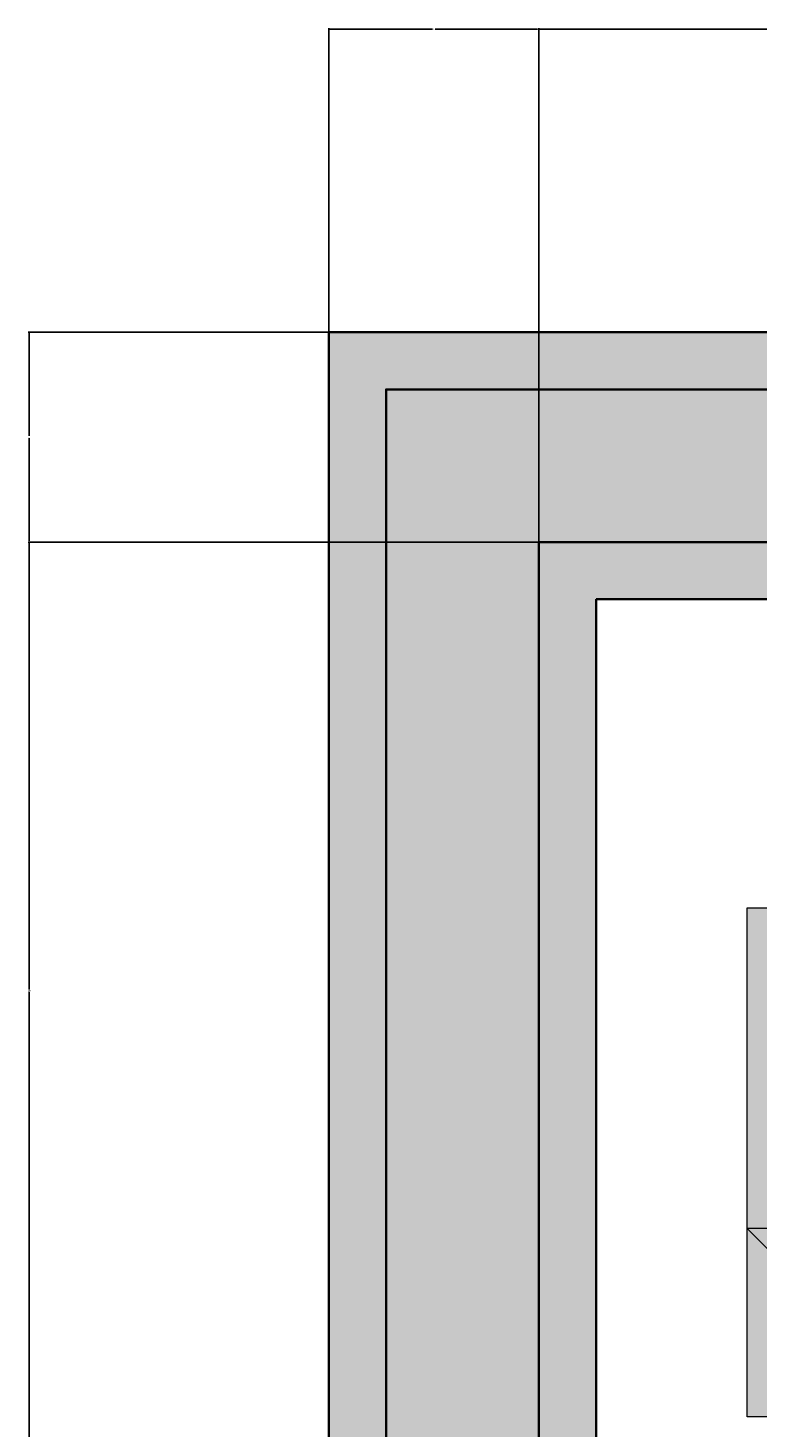
# Model space of a CAD drawing. Units: inches. Extents: x 2549 to 3108, y 1683 to 2362.
# Tile 19 of 30: x 2549 to 2664, y 2142 to 2362. Entities that reach past the tile are written whole.
import ezdxf

# ---------------------------------------------------------------- set-up
doc = ezdxf.new("R2010")
doc.units = ezdxf.units.IN
for name, color, linetype, lineweight in [('A-ANNO-DIMS', 2, 'Continuous', 18), ('A-FURN', 8, 'Continuous', 18), ('A-FURN-PATT', 9, 'Continuous', 13), ('A-WALL', 7, 'Continuous', 35), ('A-WALL-PATT', 89, 'Continuous', 13), ('C-PROP', 7, 'Continuous', 35)]:
    doc.layers.add(name, color=color, linetype=linetype, lineweight=lineweight)
for name, color, linetype, lineweight, true_color in [('C-PKNG-VEHI-PATT', 251, 'Continuous', 13, 0x636466), ('C-PROP-PATT', 252, 'Continuous', 13, 0x939598), ('C-PVMT-PATT', 9, 'Continuous', 13, 0xc7c8ca)]:
    doc.layers.add(name, color=color, linetype=linetype, lineweight=lineweight, true_color=true_color)
doc.styles.get("Standard").update_dxf_attribs({"font": 'arial.ttf'})
doc.dimstyles.get("Standard").update_dxf_attribs({"dimtxt": 0.18, "dimasz": 0.18, "dimexe": 0.18, "dimexo": 0.0625, "dimgap": 0.09, "dimtad": 0, "dimtih": 1, "dimtoh": 1, "dimdec": 4, "dimzin": 0, "dimdsep": 46, "dimtxsty": 'Standard', "dimcen": 0.09, "dimadec": 0, "dimazin": 0, "dimtfac": 1, "dimtdec": 4, "dimtofl": 0, "dimtmove": 0, "dimatfit": 3, "dimfxl": 1, "dimtolj": 1, "dimtzin": 0, "dimarcsym": 0})

# ---------------------------------------------------------------- blocks, each defined once
blk = doc.blocks.new('Bed - Queen')
for p, q in [((0, -80.00003), (0, 0)), ((0, 0), (59.99999, 0)), ((59.99999, 0), (59.99999, -80.00003)), ((7.99999, -1.2), (28.79998, -1.2)), ((7.99999, -14.4), (7.99999, -1.2)), ((28.79998, -1.2), (28.79998, -14.4)), ((31.19999, -1.2), (51.99999, -1.2)), ((31.19999, -14.4), (31.19999, -1.2)), ((51.99999, -1.2), (51.99999, -16.4)), ((0, -14.4), (44.8, -14.4)), ((59.99999, -29.6), (44.8, -14.4)), ((44.8, -14.4), (44.8, -29.6)), ((44.8, -16.8), (0, -16.8)), ((51.99999, -16.4), (46.79936, -16.4)), ((44.8, -29.6), (59.99999, -29.6)), ((59.99999, -80.00003), (0, -80.00003))]:
    blk.add_line(p, q)
blk = doc.blocks.new('*D26')
at = {"layer": 'A-ANNO-DIMS', "color": 0, "lineweight": -2, "transparency": 16777216}
for p, q in [((2596.64, 2314.59), (2596.64, 2362.32)), ((2596.82, 2362.14), (2612.92, 2362.14)), ((2629.46, 2362.14), (2613.36, 2362.14)), ((2629.64, 2281.59), (2629.64, 2362.32))]:
    blk.add_line(p, q, dxfattribs=at)
at = {"layer": 'A-ANNO-DIMS', "color": 0, "transparency": 16777216}
for points in [[(2596.82, 2362.17), (2596.82, 2362.11), (2596.64, 2362.14)], [(2629.46, 2362.17), (2629.46, 2362.11), (2629.64, 2362.14)]]:
    blk.add_solid(points, dxfattribs=at)
at = {"layer": 'Defpoints', "color": 0, "transparency": 16777216}
for p in [(2629.64, 2362.14), (2596.64, 2314.52), (2629.64, 2281.52)]:
    blk.add_point(p, dxfattribs=at)
at = {"layer": 'A-ANNO-DIMS', "color": 0, "transparency": 16777216, "insert": (2613.14, 2362.14), "char_height": 0.18, "attachment_point": 5}
blk.add_mtext('\\A1;33', dxfattribs=at)
blk = doc.blocks.new('*D27')
at = {"layer": 'A-ANNO-DIMS', "color": 0, "lineweight": -2, "transparency": 16777216}
for p, q in [((2629.64, 2281.59), (2629.64, 2362.32)), ((2629.82, 2362.14), (2720.86, 2362.14)), ((2812.46, 2362.14), (2721.42, 2362.14)), ((2812.64, 2272.59), (2812.64, 2362.32))]:
    blk.add_line(p, q, dxfattribs=at)
at = {"layer": 'A-ANNO-DIMS', "color": 0, "transparency": 16777216}
for points in [[(2629.82, 2362.17), (2629.82, 2362.11), (2629.64, 2362.14)], [(2812.46, 2362.17), (2812.46, 2362.11), (2812.64, 2362.14)]]:
    blk.add_solid(points, dxfattribs=at)
at = {"layer": 'Defpoints', "color": 0, "transparency": 16777216}
for p in [(2812.64, 2362.14), (2629.64, 2281.52), (2812.64, 2272.52)]:
    blk.add_point(p, dxfattribs=at)
at = {"layer": 'A-ANNO-DIMS', "color": 0, "transparency": 16777216, "insert": (2721.14, 2362.14), "char_height": 0.18, "attachment_point": 5}
blk.add_mtext('\\A1;183', dxfattribs=at)
blk = doc.blocks.new('*D31')
at = {"layer": 'A-ANNO-DIMS', "color": 0, "lineweight": -2, "transparency": 16777216}
for p, q in [((2596.58, 2314.52), (2549.42, 2314.52)), ((2549.6, 2314.34), (2549.6, 2298.21)), ((2549.6, 2281.7), (2549.6, 2297.84)), ((2629.58, 2281.52), (2549.42, 2281.52))]:
    blk.add_line(p, q, dxfattribs=at)
at = {"layer": 'A-ANNO-DIMS', "color": 0, "transparency": 16777216}
for points in [[(2549.57, 2314.34), (2549.63, 2314.34), (2549.6, 2314.52)], [(2549.57, 2281.7), (2549.63, 2281.7), (2549.6, 2281.52)]]:
    blk.add_solid(points, dxfattribs=at)
at = {"layer": 'Defpoints', "color": 0, "transparency": 16777216}
for p in [(2549.6, 2314.52), (2596.64, 2314.52), (2629.64, 2281.52)]:
    blk.add_point(p, dxfattribs=at)
at = {"layer": 'A-ANNO-DIMS', "color": 0, "transparency": 16777216, "insert": (2549.6, 2298.02), "char_height": 0.18, "attachment_point": 5}
blk.add_mtext('\\A1;33', dxfattribs=at)
blk = doc.blocks.new('*D32')
at = {"layer": 'A-ANNO-DIMS', "color": 0, "lineweight": -2, "transparency": 16777216}
for p, q in [((2629.58, 2281.52), (2549.42, 2281.52)), ((2549.6, 2281.34), (2549.6, 2211.2)), ((2549.6, 2140.7), (2549.6, 2210.84)), ((2638.58, 2140.52), (2549.42, 2140.52))]:
    blk.add_line(p, q, dxfattribs=at)
at = {"layer": 'A-ANNO-DIMS', "color": 0, "transparency": 16777216}
for points in [[(2549.57, 2281.34), (2549.63, 2281.34), (2549.6, 2281.52)], [(2549.57, 2140.7), (2549.63, 2140.7), (2549.6, 2140.52)]]:
    blk.add_solid(points, dxfattribs=at)
at = {"layer": 'Defpoints', "color": 0, "transparency": 16777216}
for p in [(2549.6, 2281.52), (2629.64, 2281.52), (2638.64, 2140.52)]:
    blk.add_point(p, dxfattribs=at)
at = {"layer": 'A-ANNO-DIMS', "color": 0, "transparency": 16777216, "insert": (2549.6, 2211.02), "char_height": 0.18, "attachment_point": 5}
blk.add_mtext('\\A1;141', dxfattribs=at)

msp = doc.modelspace()

# ---------------------------------------------------------------- hatches: boundary and pattern name
at = {"layer": 'A-FURN-PATT', "transparency": 33554567}
h = msp.add_hatch(color=256, dxfattribs=at)
h.dxf.hatch_style = 1
h.paths.add_polyline_path([(2708.7147, 2271.6737), (2675.2813, 2271.6737), (2675.2813, 2262.0404), (2708.7147, 2262.0404)])
h.paths.add_polyline_path([(2980.8246, 2271.6737), (2947.3913, 2271.6737), (2947.3913, 2262.0404), (2980.8246, 2262.0404)])
h.paths.add_polyline_path([(2748.8496, 2101.6383), (2798.148, 2101.6383), (2798.148, 2111.4248), (2748.8496, 2111.4248)], flags=9)
h.paths.add_polyline_path([(2685.2081, 2101.489), (2719.3253, 2101.489), (2719.3253, 2111.2819), (2685.2081, 2111.2819)], flags=9)
h.paths.add_polyline_path([(2814.6852, 1907.1328), (2847.8384, 1907.1328), (2847.8384, 1916.9258), (2814.6852, 1916.9258)], flags=9)
h.paths.add_polyline_path([(2814.3906, 1835.5864), (2848.0172, 1835.5864), (2848.0172, 1845.3794), (2814.3906, 1845.3794)], flags=9)
h.paths.add_polyline_path([(2800.5245, 1759.1674), (2853.7435, 1759.1674), (2853.7435, 1768.954), (2800.5245, 1768.954)], flags=9)
h.paths.add_polyline_path([(2972.4611, 1807.3305), (3015.3943, 1807.3305), (3015.3943, 1817.117), (2972.4611, 1817.117)], flags=9)
h.paths.add_polyline_path([(2902.3327, 1888.6731), (2937.9131, 1888.6731), (2937.9131, 1898.4661), (2902.3327, 1898.4661)], flags=9)
h.paths.add_polyline_path([(2712.1779, 1878.9039), (2754.1257, 1878.9039), (2754.1257, 1888.6904), (2712.1779, 1888.6904)], flags=9)
h.paths.add_polyline_path([(2614.0056, 2012.812), (2650.0251, 2012.812), (2650.0251, 2022.4371), (2614.0056, 2022.4371)], flags=9)
h.paths.add_polyline_path([(2713.3129, 2003.1645), (2747.4237, 2003.1645), (2747.4237, 2012.951), (2713.3129, 2012.951)], flags=9)
h.paths.add_polyline_path([(2950.1379, 2001.6934), (2982.2992, 2001.6934), (2982.2992, 2011.48), (2950.1379, 2011.48)], flags=9)
h.paths.add_polyline_path([(2940.864, 2238.5537), (2997.5066, 2238.5537), (2997.5066, 2248.3466), (2940.864, 2248.3466)], flags=9)
h.paths.add_polyline_path([(2821.5457, 2202.8348), (2855.663, 2202.8348), (2855.663, 2212.6278), (2821.5457, 2212.6278)], flags=9)
h.paths.add_polyline_path([(2661.8026, 2238.6249), (2718.4451, 2238.6249), (2718.4451, 2248.4179), (2661.8026, 2248.4179)], flags=9)
h = msp.add_hatch(color=256, dxfattribs=at)
h.dxf.hatch_style = 1
h.paths.add_polyline_path([(2906.5064, 1905.2148), (2905.2584, 1904.3827), (2907.0611, 1900.7772), (2908.3092, 1901.6092)])
h.paths.add_polyline_path([(2936.522, 1914.8044), (2935.2739, 1915.6364), (2932.6391, 1912.5856), (2933.8871, 1911.7535)])
h.paths.add_polyline_path([(2950.2508, 1905.6518), (2949.0027, 1906.4839), (2947.1999, 1902.8783), (2948.448, 1902.0463)])
h.paths.add_polyline_path([(2958.5713, 1918.1326), (2956.9072, 1919.242), (2952.4696, 1908.98, 1.38742744), (2954.9657, 1907.3159)])
h.paths.add_polyline_path([(2945.2585, 1927.0078), (2943.5944, 1928.1172), (2934.9965, 1920.6287, 1.38742744), (2937.4927, 1918.9646)])
h.paths.add_polyline_path([(2748.8496, 2101.6383), (2798.148, 2101.6383), (2798.148, 2111.4248), (2748.8496, 2111.4248)], flags=9)
h.paths.add_polyline_path([(2685.2081, 2101.489), (2719.3253, 2101.489), (2719.3253, 2111.2819), (2685.2081, 2111.2819)], flags=9)
h.paths.add_polyline_path([(2814.6852, 1907.1328), (2847.8384, 1907.1328), (2847.8384, 1916.9258), (2814.6852, 1916.9258)], flags=9)
h.paths.add_polyline_path([(2814.3906, 1835.5864), (2848.0172, 1835.5864), (2848.0172, 1845.3794), (2814.3906, 1845.3794)], flags=9)
h.paths.add_polyline_path([(2800.5245, 1759.1674), (2853.7435, 1759.1674), (2853.7435, 1768.954), (2800.5245, 1768.954)], flags=9)
h.paths.add_polyline_path([(2972.4611, 1807.3305), (3015.3943, 1807.3305), (3015.3943, 1817.117), (2972.4611, 1817.117)], flags=9)
h.paths.add_polyline_path([(2902.3327, 1888.6731), (2937.9131, 1888.6731), (2937.9131, 1898.4661), (2902.3327, 1898.4661)], flags=9)
h.paths.add_polyline_path([(2712.1779, 1878.9039), (2754.1257, 1878.9039), (2754.1257, 1888.6904), (2712.1779, 1888.6904)], flags=9)
h.paths.add_polyline_path([(2614.0056, 2012.812), (2650.0251, 2012.812), (2650.0251, 2022.4371), (2614.0056, 2022.4371)], flags=9)
h.paths.add_polyline_path([(2713.3129, 2003.1645), (2747.4237, 2003.1645), (2747.4237, 2012.951), (2713.3129, 2012.951)], flags=9)
h.paths.add_polyline_path([(2950.1379, 2001.6934), (2982.2992, 2001.6934), (2982.2992, 2011.48), (2950.1379, 2011.48)], flags=9)
h.paths.add_polyline_path([(2940.864, 2238.5537), (2997.5066, 2238.5537), (2997.5066, 2248.3466), (2940.864, 2248.3466)], flags=9)
h.paths.add_polyline_path([(2821.5457, 2202.8348), (2855.663, 2202.8348), (2855.663, 2212.6278), (2821.5457, 2212.6278)], flags=9)
h.paths.add_polyline_path([(2661.8026, 2238.6249), (2718.4451, 2238.6249), (2718.4451, 2248.4179), (2661.8026, 2248.4179)], flags=9)
at = {"layer": 'A-FURN-PATT', "transparency": 33554684}
h = msp.add_hatch(color=256, dxfattribs=at)
h.dxf.hatch_style = 1
h.paths.add_polyline_path([(2722.3589, 2224.0179), (2662.3589, 2224.0179), (2662.3589, 2173.6179), (2677.5589, 2173.6179), (2677.5589, 2160.8179), (2722.3589, 2160.8179)])
h.paths.add_polyline_path([(2996.4972, 2224.0179), (2936.4972, 2224.0179), (2936.4972, 2173.6179), (2951.6972, 2173.6179), (2951.6972, 2160.8179), (2996.4972, 2160.8179)])
h = msp.add_hatch(color=256, dxfattribs=at)
h.dxf.hatch_style = 1
h.paths.add_polyline_path([(2677.5589, 2173.6179), (2662.3589, 2173.6179), (2677.5589, 2158.4179)], flags=17)
h.paths.add_polyline_path([(2662.3589, 2173.6179), (2662.3589, 2144.0179), (2722.3589, 2144.0179), (2722.3589, 2158.4179), (2714.3589, 2158.4179), (2714.3589, 2145.2179), (2693.5589, 2145.2179), (2693.5589, 2158.4179), (2691.1589, 2158.4179), (2691.1589, 2145.2179), (2670.3589, 2145.2179), (2670.3589, 2160.4179), (2675.5589, 2160.4179)])
h.paths.add_polyline_path([(2722.3589, 2160.8179), (2677.5589, 2160.8179), (2677.5589, 2158.4179), (2722.3589, 2158.4179)], flags=17)
h.paths.add_polyline_path([(2951.6972, 2173.6179), (2936.4972, 2173.6179), (2951.6972, 2158.4179)], flags=17)
h.paths.add_polyline_path([(2936.4972, 2173.6179), (2936.4972, 2144.0179), (2996.4972, 2144.0179), (2996.4972, 2158.4179), (2988.4972, 2158.4179), (2988.4972, 2145.2179), (2967.6972, 2145.2179), (2967.6972, 2158.4179), (2965.2972, 2158.4179), (2965.2972, 2145.2179), (2944.4972, 2145.2179), (2944.4972, 2160.4179), (2949.6972, 2160.4179)])
h.paths.add_polyline_path([(2996.4972, 2160.8179), (2951.6972, 2160.8179), (2951.6972, 2158.4179), (2996.4972, 2158.4179)], flags=17)
at = {"layer": 'A-WALL-PATT'}
h = msp.add_hatch(color=256, dxfattribs=at)
h.dxf.hatch_style = 1
h.paths.add_polyline_path([(2638.6427, 2272.5237), (3034.6427, 2272.5237), (3034.6427, 1936.5237), (3043.6427, 1936.5237), (3043.6427, 2281.5237), (2629.6427, 2281.5237), (2629.6427, 2074.5237), (2812.6427, 2074.5237), (2812.6427, 2140.5237), (2785.7177, 2140.5237), (2785.7177, 2134.5237), (2806.6427, 2134.5237), (2806.6427, 2080.5237), (2638.6427, 2080.5237)])
h.paths.add_polyline_path([(2638.6427, 1972.5237), (2662.6427, 1972.5237), (2662.6427, 2041.0557), (2653.6427, 2041.0557), (2653.6427, 1978.5237), (2629.6427, 1978.5237), (2629.6427, 1795.5237), (2662.6427, 1795.5237), (2881.6427, 1795.5237), (2881.6427, 1936.5237), (2965.9351, 1936.5237), (2965.9351, 1974.5439), (2959.9351, 1974.5439), (2959.9351, 1945.5237), (2881.6427, 1945.5237), (2872.6427, 1945.5237), (2872.6427, 1804.5237), (2662.6427, 1804.5237), (2638.6427, 1804.5237)])
at = {"layer": 'C-PKNG-VEHI-PATT'}
h = msp.add_hatch(color=256, dxfattribs=at)
h.dxf.hatch_style = 1
edge = h.paths.add_edge_path()
edge.add_ellipse((2935.7258, 1791.964), major_axis=(-50.66, 0), ratio=0.84230387, start_angle=248.165046, end_angle=265.722579)
edge.add_line((2938.911, 1834.5507), (2925.8653, 1834.5507))
edge.add_ellipse((2929.0505, 1791.964), major_axis=(50.66, 0), ratio=0.84230387, start_angle=94.277421, end_angle=111.834954)
edge.add_line((2912.8508, 1832.3947), (2914.2044, 1822.2495))
edge.add_ellipse((2930.6538, 1783.1023), major_axis=(-49.3014, 0), ratio=0.84230387, start_angle=-85.12993, end_angle=-67.208085, ccw=False)
edge.add_line((2927.1247, 1824.5225), (2937.6516, 1824.5225))
edge.add_ellipse((2934.1225, 1783.1023), major_axis=(49.3014, 0), ratio=0.84230387, start_angle=67.208085, end_angle=85.12993, ccw=False)
edge.add_line((2950.5719, 1822.2495), (2951.9255, 1832.3947))
edge = h.paths.add_edge_path()
edge.add_ellipse((2903.4793, 1857.3351), major_axis=(-34.7979, 0), ratio=0.84230387, start_angle=180, end_angle=209.43857)
edge.add_ellipse((2961.297, 1857.3351), major_axis=(34.7979, 0), ratio=0.84230387, start_angle=150.56143, end_angle=180)
edge.add_line((2926.4991, 1857.3351), (2926.4991, 1843.7609))
edge.add_ellipse((2924.1251, 1844.3143), major_axis=(-0.2209, 3.9278), ratio=0.60383358, start_angle=89.002014, end_angle=253.657408, ccw=False)
edge.add_line((2921.7512, 1844.2222), (2921.7512, 1853.3975))
edge.add_line((2921.7512, 1853.3975), (2925.269, 1855.8484))
edge.add_ellipse((2925.4782, 1855.4931), major_axis=(0.4584, 0), ratio=0.84230387, start_angle=90, end_angle=134.480211, ccw=False)
edge.add_line((2925.4782, 1855.8792), (2926.4991, 1855.8792))
edge.add_line((2926.4991, 1855.8792), (2926.4991, 1857.3351))
edge.add_ellipse((2961.297, 1857.3351), major_axis=(34.7979, 0), ratio=0.84230387, start_angle=150.56143, end_angle=180, ccw=False)
edge.add_line((2932.3882, 1873.6501), (2932.3882, 1875.7801))
edge.add_ellipse((2932.3882, 1875.3939), major_axis=(0.4584, 0), ratio=0.84230387, start_angle=90, end_angle=127.93313)
edge.add_line((2932.1366, 1875.7167), (2928.5915, 1873.7564))
edge.add_ellipse((2899.9271, 2002.4692), major_axis=(155.4756, 0), ratio=0.84230387, start_angle=-80.743434, end_angle=-77.445067, ccw=False)
edge.add_ellipse((2949.4402, 1715.2151), major_axis=(-189.1422, 0), ratio=0.84230387, start_angle=-79.790461, end_angle=-77.555373)
edge.add_ellipse((3300.3614, 1852.5642), major_axis=(-386.1662, 0), ratio=0.84230387, start_angle=-2.863715, end_angle=2.198541)
edge.add_ellipse((2929.0505, 1792.5159), major_axis=(-55.6192, 0), ratio=0.84230387, start_angle=-85.917589, end_angle=-72.280047, ccw=False)
edge.add_line((2925.7129, 1839.2798), (2939.0634, 1839.2798))
edge.add_ellipse((2935.7258, 1792.5159), major_axis=(55.6192, 0), ratio=0.84230387, start_angle=72.280047, end_angle=85.917589, ccw=False)
edge.add_ellipse((2564.4149, 1852.5642), major_axis=(-386.1662, 0), ratio=0.84230387, start_angle=177.801459, end_angle=182.863715)
edge.add_ellipse((2915.3361, 1715.2151), major_axis=(189.1422, 0), ratio=0.84230387, start_angle=77.555373, end_angle=79.790461)
edge.add_ellipse((2964.8492, 2002.4692), major_axis=(-155.4756, 0), ratio=0.84230387, start_angle=77.445067, end_angle=80.743434, ccw=False)
edge.add_line((2936.1848, 1873.7564), (2932.6397, 1875.7167))
edge.add_ellipse((2932.3882, 1875.3939), major_axis=(0.4584, 0), ratio=0.84230387, start_angle=52.06687, end_angle=90)
edge.add_line((2932.3882, 1875.7801), (2932.3882, 1873.6501))
edge.add_ellipse((2903.4793, 1857.3351), major_axis=(-34.7979, 0), ratio=0.84230387, start_angle=180, end_angle=209.43857, ccw=False)
edge.add_line((2938.2772, 1857.3351), (2938.2772, 1855.8792))
edge.add_line((2938.2772, 1855.8792), (2939.4059, 1855.8792))
edge.add_ellipse((2939.2981, 1855.4931), major_axis=(-0.4584, 0), ratio=0.84230387, start_angle=225.519789, end_angle=270, ccw=False)
edge.add_line((2939.5903, 1855.7906), (2943.0251, 1853.3975))
edge.add_line((2943.0251, 1853.3975), (2943.0251, 1844.2222))
edge.add_ellipse((2940.6512, 1844.3143), major_axis=(0.2209, 3.9278), ratio=0.60383358, start_angle=106.342592, end_angle=270.997986, ccw=False)
edge.add_line((2938.2772, 1843.7609), (2938.2772, 1857.3351))
edge = h.paths.add_edge_path()
edge.add_ellipse((2932.3882, 1865.1973), major_axis=(91.081, 0), ratio=0.84230387, start_angle=256.401865, end_angle=283.598135, ccw=False)
edge.add_line((2914.2044, 1790.0239), (2914.2044, 1778.3622))
edge.add_ellipse((2932.3882, 1853.5356), major_axis=(91.081, 0), ratio=0.84230387, start_angle=256.401865, end_angle=283.598135)
edge.add_line((2950.5719, 1778.3622), (2950.5719, 1790.0239))
edge = h.paths.add_edge_path()
edge.add_ellipse((2948.7383, 1772.3145), major_axis=(1.8336, 0), ratio=0.84230387, start_angle=0, end_angle=90)
edge.add_line((2948.7383, 1773.859), (2916.038, 1773.859))
edge.add_ellipse((2916.038, 1772.3145), major_axis=(1.8336, 0), ratio=0.84230387, start_angle=90, end_angle=180)
edge.add_line((2914.2044, 1772.3145), (2914.2044, 1760.2558))
edge.add_line((2914.2044, 1760.2558), (2950.5719, 1760.2558))
edge.add_line((2950.5719, 1760.2558), (2950.5719, 1772.3145))
h.paths.add_polyline_path([(2748.8496, 2101.6383), (2798.148, 2101.6383), (2798.148, 2111.4248), (2748.8496, 2111.4248)], flags=9)
h.paths.add_polyline_path([(2685.2081, 2101.489), (2719.3253, 2101.489), (2719.3253, 2111.2819), (2685.2081, 2111.2819)], flags=9)
h.paths.add_polyline_path([(2814.6852, 1907.1328), (2847.8384, 1907.1328), (2847.8384, 1916.9258), (2814.6852, 1916.9258)], flags=9)
h.paths.add_polyline_path([(2814.3906, 1835.5864), (2848.0172, 1835.5864), (2848.0172, 1845.3794), (2814.3906, 1845.3794)], flags=9)
h.paths.add_polyline_path([(2800.5245, 1759.1674), (2853.7435, 1759.1674), (2853.7435, 1768.954), (2800.5245, 1768.954)], flags=9)
h.paths.add_polyline_path([(2972.4611, 1807.3305), (3015.3943, 1807.3305), (3015.3943, 1817.117), (2972.4611, 1817.117)], flags=9)
h.paths.add_polyline_path([(2902.3327, 1888.6731), (2937.9131, 1888.6731), (2937.9131, 1898.4661), (2902.3327, 1898.4661)], flags=9)
h.paths.add_polyline_path([(2712.1779, 1878.9039), (2754.1257, 1878.9039), (2754.1257, 1888.6904), (2712.1779, 1888.6904)], flags=9)
h.paths.add_polyline_path([(2614.0056, 2012.812), (2650.0251, 2012.812), (2650.0251, 2022.4371), (2614.0056, 2022.4371)], flags=9)
h.paths.add_polyline_path([(2713.3129, 2003.1645), (2747.4237, 2003.1645), (2747.4237, 2012.951), (2713.3129, 2012.951)], flags=9)
h.paths.add_polyline_path([(2950.1379, 2001.6934), (2982.2992, 2001.6934), (2982.2992, 2011.48), (2950.1379, 2011.48)], flags=9)
h.paths.add_polyline_path([(2940.864, 2238.5537), (2997.5066, 2238.5537), (2997.5066, 2248.3466), (2940.864, 2248.3466)], flags=9)
h.paths.add_polyline_path([(2821.5457, 2202.8348), (2855.663, 2202.8348), (2855.663, 2212.6278), (2821.5457, 2212.6278)], flags=9)
h.paths.add_polyline_path([(2661.8026, 2238.6249), (2718.4451, 2238.6249), (2718.4451, 2248.4179), (2661.8026, 2248.4179)], flags=9)
at = {"layer": 'C-PROP-PATT'}
h = msp.add_hatch(color=256, dxfattribs=at)
h.dxf.hatch_style = 1
h.paths.add_polyline_path([(3076.6427, 2314.5237), (2596.6427, 2314.5237), (2596.6427, 1714.5237), (2881.84, 1714.5237), (2881.84, 1723.5237), (2605.6427, 1723.5237), (2605.6427, 2305.5237), (3067.6427, 2305.5237), (3067.6427, 1723.5237), (3067.6427, 1714.5237), (3076.6427, 1714.5237)])
at = {"layer": 'C-PVMT-PATT'}
h = msp.add_hatch(color=256, dxfattribs=at)
h.dxf.hatch_style = 1
h.paths.add_polyline_path([(3067.6427, 2305.5237), (2605.6427, 2305.5237), (2605.6427, 2074.5237), (2629.6427, 2074.5237), (2629.6427, 2281.5237), (3043.6427, 2281.5237), (3043.6427, 1885.5237), (3043.6427, 1872.8745), (3031.1672, 1872.8745), (3031.1672, 1862.5731), (2995.8054, 1862.5731), (2995.8054, 1872.8745), (2983.1752, 1872.8745), (2983.1752, 1885.5237), (2881.6427, 1885.5237), (2881.6427, 1795.5237), (2751.0977, 1795.5237), (2751.0977, 1761.5237), (2786.1577, 1761.5237), (2786.1577, 1723.5237), (2881.84, 1723.5237), (2881.84, 1714.5237), (3067.6427, 1714.5237), (3067.6427, 1723.5237)])
edge = h.paths.add_edge_path(flags=16)
edge.add_ellipse((2949.4402, 1710.9683), major_axis=(-194.1014, 0), ratio=0.84230387, start_angle=-77.874034, end_angle=-76.219471, ccw=False)
edge.add_ellipse((2949.4402, 1715.2151), major_axis=(-189.1422, 0), ratio=0.84230387, start_angle=-79.790461, end_angle=-77.555373, ccw=False)
edge.add_ellipse((2899.9271, 2002.4692), major_axis=(155.4756, 0), ratio=0.84230387, start_angle=-80.743434, end_angle=-77.445067)
edge.add_line((2928.5915, 1873.7564), (2932.3882, 1875.8558))
edge.add_line((2932.3882, 1875.8558), (2936.1848, 1873.7564))
edge.add_ellipse((2964.8492, 2002.4692), major_axis=(-155.4756, 0), ratio=0.84230387, start_angle=77.445067, end_angle=80.743434)
edge.add_ellipse((2915.3361, 1715.2151), major_axis=(189.1422, 0), ratio=0.84230387, start_angle=77.555373, end_angle=79.790461, ccw=False)
edge.add_ellipse((2915.3361, 1710.9683), major_axis=(-194.1014, 0), ratio=0.84230387, start_angle=256.219471, end_angle=257.874034, ccw=False)
edge.add_ellipse((2628.2871, 1850.2612), major_axis=(-327.2532, 0), ratio=0.84230387, start_angle=182.17995, end_angle=183.650428, ccw=False)
edge.add_ellipse((2955.5637, 1861.9334), major_axis=(-0.9168, 0), ratio=0.84230387, start_angle=180, end_angle=270, ccw=False)
edge.add_line((2956.4805, 1862.3857), (2956.4805, 1846.4866))
edge.add_ellipse((2955.5637, 1846.939), major_axis=(-0.9168, 0), ratio=0.84230387, start_angle=90, end_angle=180, ccw=False)
edge.add_ellipse((-3607.0606, 1835.832), major_axis=(-6562.6242, 0), ratio=0.84230387, start_angle=179.61613322, end_angle=180.09022909, ccw=False)
edge.add_ellipse((2955.5637, 1791.0926), major_axis=(0.9168, 0), ratio=0.84230387, start_angle=0, end_angle=90, ccw=False)
edge.add_line((2956.4805, 1791.545), (2956.4805, 1775.6459))
edge.add_ellipse((2955.5637, 1776.0982), major_axis=(0.9168, 0), ratio=0.84230387, start_angle=270, end_angle=360, ccw=False)
edge.add_ellipse((-3607.0606, 1835.832), major_axis=(-6562.6242, 0), ratio=0.84230387, start_angle=179.3813568, end_angle=179.47172853, ccw=False)
edge.add_ellipse((2954.5907, 1763.8768), major_axis=(-1.3752, 0), ratio=0.84230387, start_angle=179.371763, end_angle=248.464757, ccw=False)
edge.add_ellipse((-3607.519, 1835.832), major_axis=(-6564.0409, 0), ratio=0.842303863, start_angle=179.35344594, end_angle=179.37176282, ccw=False)
edge.add_ellipse((2952.6829, 1761.8002), major_axis=(3.2503, 0), ratio=0.84230387, start_angle=-90, end_angle=-0.646554, ccw=False)
edge.add_line((2952.6829, 1759.0625), (2912.0934, 1759.0625))
edge.add_ellipse((2912.0934, 1761.8002), major_axis=(3.2503, 0), ratio=0.84230387, start_angle=180.646554, end_angle=270, ccw=False)
edge.add_ellipse((9472.2953, 1835.832), major_axis=(-6564.0409, 0), ratio=0.842303871, start_angle=0.62823722, end_angle=0.6465541, ccw=False)
edge.add_ellipse((2910.1856, 1763.8768), major_axis=(1.3752, 0), ratio=0.84230387, start_angle=111.535244, end_angle=180.628237, ccw=False)
edge.add_ellipse((9471.8369, 1835.832), major_axis=(-6562.6242, 0), ratio=0.84230387, start_angle=0.52827147, end_angle=0.6465541, ccw=False)
edge.add_ellipse((2909.2126, 1776.0982), major_axis=(-0.9168, 0), ratio=0.84230387, start_angle=0, end_angle=90, ccw=False)
edge.add_line((2908.2958, 1775.6459), (2908.2958, 1791.545))
edge.add_ellipse((2909.2126, 1791.0926), major_axis=(-0.9168, 0), ratio=0.84230387, start_angle=-90, end_angle=0, ccw=False)
edge.add_ellipse((9471.8369, 1835.832), major_axis=(-6562.6242, 0), ratio=0.84230387, start_angle=-0.09022909, end_angle=0.38386678, ccw=False)
edge.add_ellipse((2909.2126, 1846.939), major_axis=(-0.9168, 0), ratio=0.84230387, start_angle=0, end_angle=90, ccw=False)
edge.add_line((2908.2958, 1846.4866), (2908.2958, 1862.3857))
edge.add_ellipse((2909.2126, 1861.9334), major_axis=(0.9168, 0), ratio=0.84230387, start_angle=90, end_angle=180, ccw=False)
edge.add_ellipse((3236.4892, 1850.2612), major_axis=(327.2532, 0), ratio=0.84230387, start_angle=176.349572, end_angle=177.82005, ccw=False)
edge = h.paths.add_edge_path(flags=0)
edge.add_ellipse((2903.4793, 1857.3351), major_axis=(-34.7979, 0), ratio=0.84230387, start_angle=180, end_angle=209.43857, ccw=False)
edge.add_line((2938.2772, 1857.3351), (2938.2772, 1855.8792))
edge.add_line((2938.2772, 1855.8792), (2939.4631, 1855.8792))
edge.add_line((2939.4631, 1855.8792), (2943.0251, 1853.3975))
edge.add_line((2943.0251, 1853.3975), (2943.0251, 1844.2222))
edge.add_ellipse((2940.6512, 1844.3143), major_axis=(0.2209, 3.9278), ratio=0.60383358, start_angle=106.342592, end_angle=270.997986, ccw=False)
edge.add_line((2938.2772, 1843.7609), (2938.2772, 1857.3351))
edge.add_ellipse((2903.4793, 1857.3351), major_axis=(-34.7979, 0), ratio=0.84230387, start_angle=180, end_angle=209.43857)
edge.add_ellipse((2961.297, 1857.3351), major_axis=(34.7979, 0), ratio=0.84230387, start_angle=150.56143, end_angle=180)
edge.add_line((2926.4991, 1857.3351), (2926.4991, 1843.7609))
edge.add_ellipse((2924.1251, 1844.3143), major_axis=(-0.2209, 3.9278), ratio=0.60383358, start_angle=89.002014, end_angle=253.657408, ccw=False)
edge.add_line((2921.7512, 1844.2222), (2921.7512, 1853.3975))
edge.add_line((2921.7512, 1853.3975), (2925.3132, 1855.8792))
edge.add_line((2925.3132, 1855.8792), (2926.4991, 1855.8792))
edge.add_line((2926.4991, 1855.8792), (2926.4991, 1857.3351))
edge.add_ellipse((2961.297, 1857.3351), major_axis=(34.7979, 0), ratio=0.84230387, start_angle=150.56143, end_angle=180, ccw=False)
edge = h.paths.add_edge_path(flags=0)
edge.add_ellipse((2929.0505, 1791.964), major_axis=(50.66, 0), ratio=0.84230387, start_angle=94.277421, end_angle=111.834954, ccw=False)
edge.add_line((2925.8653, 1834.5507), (2938.911, 1834.5507))
edge.add_ellipse((2935.7258, 1791.964), major_axis=(-50.66, 0), ratio=0.84230387, start_angle=248.165046, end_angle=265.722579, ccw=False)
edge.add_line((2951.9255, 1832.3947), (2950.5719, 1822.2495))
edge.add_ellipse((2934.1225, 1783.1023), major_axis=(49.3014, 0), ratio=0.84230387, start_angle=67.208085, end_angle=85.12993)
edge.add_line((2937.6516, 1824.5225), (2927.1247, 1824.5225))
edge.add_ellipse((2930.6538, 1783.1023), major_axis=(-49.3014, 0), ratio=0.84230387, start_angle=-85.12993, end_angle=-67.208085)
edge.add_line((2914.2044, 1822.2495), (2912.8508, 1832.3947))
edge = h.paths.add_edge_path(flags=0)
edge.add_line((2910.1338, 1829.4651), (2912.6432, 1821.2711))
edge.add_ellipse((5203.7787, 1816.4367), major_axis=(-2291.1426, 0), ratio=0.84230387, start_angle=-0.1208974, end_angle=0.3640763)
edge.add_line((2912.7012, 1801.8782), (2910.3305, 1792.5698))
edge.add_ellipse((9471.8369, 1835.832), major_axis=(-6561.7074, 0), ratio=0.84230387, start_angle=0.05559431, end_angle=0.37776419, ccw=False)
edge = h.paths.add_edge_path(flags=0)
edge.add_ellipse((-3607.0606, 1835.832), major_axis=(6561.7074, 0), ratio=0.84230387, start_angle=-0.37776419, end_angle=-0.05559431, ccw=False)
edge.add_line((2954.4458, 1792.5698), (2952.0751, 1801.8782))
edge.add_ellipse((660.9976, 1816.4367), major_axis=(2291.1426, 0), ratio=0.84230387, start_angle=-0.3640763, end_angle=0.1208974)
edge.add_line((2952.1331, 1821.2711), (2954.6425, 1829.4651))
edge = h.paths.add_edge_path(flags=0)
edge.add_ellipse((2932.3882, 1865.1973), major_axis=(91.081, 0), ratio=0.84230387, start_angle=256.401865, end_angle=283.598135)
edge.add_line((2950.5719, 1790.0239), (2950.5719, 1778.3622))
edge.add_ellipse((2932.3882, 1853.5356), major_axis=(91.081, 0), ratio=0.84230387, start_angle=256.401865, end_angle=283.598135, ccw=False)
edge.add_line((2914.2044, 1778.3622), (2914.2044, 1790.0239))
edge = h.paths.add_edge_path(flags=0)
edge.add_line((2916.038, 1773.859), (2948.7383, 1773.859))
edge.add_ellipse((2948.7383, 1772.3145), major_axis=(1.8336, 0), ratio=0.84230387, start_angle=0, end_angle=90, ccw=False)
edge.add_line((2950.5719, 1772.3145), (2950.5719, 1760.2558))
edge.add_line((2950.5719, 1760.2558), (2914.2044, 1760.2558))
edge.add_line((2914.2044, 1760.2558), (2914.2044, 1772.3145))
edge.add_ellipse((2916.038, 1772.3145), major_axis=(1.8336, 0), ratio=0.84230387, start_angle=90, end_angle=180, ccw=False)
h.paths.add_polyline_path([(2629.6427, 1978.5237), (2605.6427, 1978.5237), (2605.6427, 1723.5237), (2629.6427, 1723.5237), (2629.6427, 1795.5237)], flags=17)
h.paths.add_polyline_path([(2800.5245, 1759.1674), (2853.7435, 1759.1674), (2853.7435, 1768.954), (2800.5245, 1768.954)], flags=24)
h.paths.add_polyline_path([(2972.4611, 1807.3305), (3015.3943, 1807.3305), (3015.3943, 1817.117), (2972.4611, 1817.117)], flags=24)

# ---------------------------------------------------------------- linework, layer by layer
at = {"layer": 'A-WALL'}
for p, q in [((2629.6427, 2281.5237), (3043.6427, 2281.5237)), ((2629.6427, 2074.5237), (2629.6427, 2281.5237)), ((2638.6427, 2272.5237), (3034.6427, 2272.5237)), ((2638.6427, 2080.5237), (2638.6427, 2272.5237))]:
    msp.add_line(p, q, dxfattribs=at)
at = {"layer": 'C-PROP'}
msp.add_lwpolyline([(2596.6427, 2314.5237), (3076.6427, 2314.5237), (3076.6427, 1714.5237), (2596.6427, 1714.5237)], close=True, dxfattribs=at)
msp.add_lwpolyline([(2881.84, 1723.5237), (2605.6427, 1723.5237), (2605.6427, 2305.5237), (3067.6427, 2305.5237), (3067.6427, 1723.5237)], dxfattribs=at)

# ---------------------------------------------------------------- block references
at = {"layer": 'A-FURN', "rotation": 180}
msp.add_blockref('Bed - Queen', (2722.3589, 2144.0179), dxfattribs=at)

# ---------------------------------------------------------------- dimensions: what is measured, and where the dimension line sits
at = {"layer": 'A-ANNO-DIMS'}
for base, p1, p2, picture, middle in [((2629.6427, 2362.1425), (2596.6427, 2314.5237), (2629.6427, 2281.5237), '*D26', (2613.1427, 2362.1425)), ((2812.6427, 2362.1425), (2629.6427, 2281.5237), (2812.6427, 2272.5237), '*D27', (2721.1427, 2362.1425))]:
    dim = msp.add_linear_dim(base=base, p1=p1, p2=p2, dimstyle='Standard', override={"dimdec": 0, "dimlfac": 1, "dimrnd": 0, "dimzin": 0, "dimdsep": 46, "dimlunit": 2}, dxfattribs=at)
    dim.commit()
    dim.dimension.update_dxf_attribs({"geometry": picture, "text_midpoint": middle})
for base, p1, p2, picture, middle in [((2549.6048, 2314.5237), (2629.6427, 2281.5237), (2596.6427, 2314.5237), '*D31', (2549.6048, 2298.0237)), ((2549.6048, 2281.5237), (2638.6427, 2140.5237), (2629.6427, 2281.5237), '*D32', (2549.6048, 2211.0237))]:
    dim = msp.add_linear_dim(base=base, p1=p1, p2=p2, angle=90, dimstyle='Standard', override={"dimdec": 0, "dimlfac": 1, "dimrnd": 0, "dimzin": 0, "dimdsep": 46, "dimlunit": 2}, dxfattribs=at)
    dim.commit()
    dim.dimension.update_dxf_attribs({"geometry": picture, "text_midpoint": middle})

doc.saveas('drawing.dxf')
